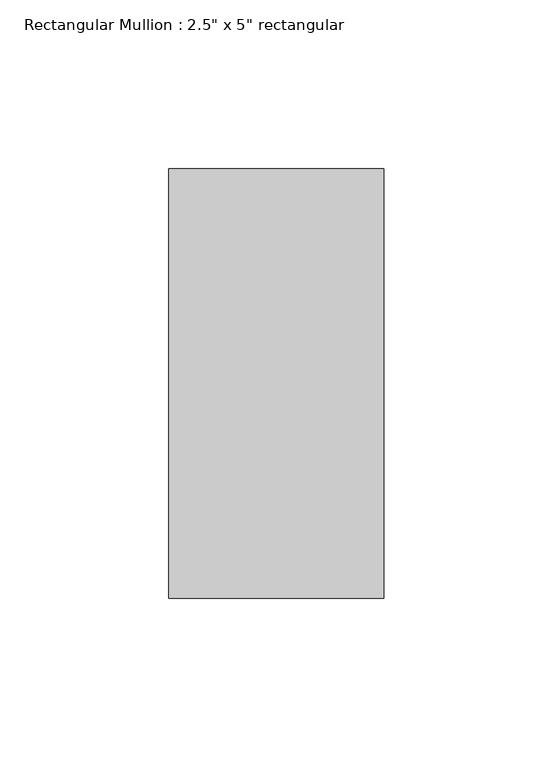
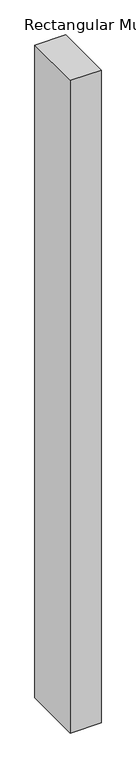
"""IFC4 building model written with IfcOpenShell, lengths in millimetres: member geometry."""

from ifc_helpers import new_model, si_unit, frame, origin, place, context, project, spatial, polyline, outline, extrude, source, transform, mapped, element, save


def member_0514ece2(model_context):
    return source(origin(), model_context, "Body", "SweptSolid", [
        extrude(outline(polyline([(31.75, 63.5), (31.75, -63.5), (-31.75, -63.5), (-31.75, 63.5), (31.75, 63.5)])), frame((0.0, 0.0, -1428.1991558), z_axis=(0.0, 0.0, 1.0), x_axis=(1.0, 0.0, 0.0)), (0.0, 0.0, 1.0), 1428.1991558),
    ])


if __name__ == "__main__":
    model = new_model("IFC4")
    model_context = context("Model", 3, world=origin())
    ifc_project = project(units=[si_unit("LENGTHUNIT", "METRE", prefix="MILLI")], contexts=[model_context])
    site = spatial("IfcSite", under=ifc_project)
    building = spatial("IfcBuilding", under=site)
    placement = place(None, origin())
    member_shape = member_0514ece2(model_context)
    element("IfcMember", 1, ObjectType="Rectangular Mullion : 2.5\" x 5\" rectangular", at=placement, inside=building, context=model_context, shape_type="MappedRepresentation", body=[
        mapped(member_shape, transform((0.0, 0.0, 0.0), x_axis=(1.0, 0.0, 0.0), y_axis=(0.0, 1.0, 0.0), z_axis=(0.0, 0.0, 1.0))),
    ])
    save(model, "model.ifc")

# Revit data of these elements
# Type "Rectangular Mullion : 2.5\" x 5\" rectangular"
#   built-in parameter 1007304 = 0.416667 (stored number, unit not read)
#   built-in parameter 1007301 = 0.104167 (stored number, unit not read)
#   built-in parameter 1007300 = 0.104167 (stored number, unit not read)
# Element 1 (IfcMember, "Rectangular Mullion : 2.5\" x 5\" rectangular")
#   Materials on its faces: "Aluminum"
# Materials
#   "Aluminum": class "Metal", colour RGB 247 247 247, transparency 0, Description = "Aluminum 6061", Cost = 0
